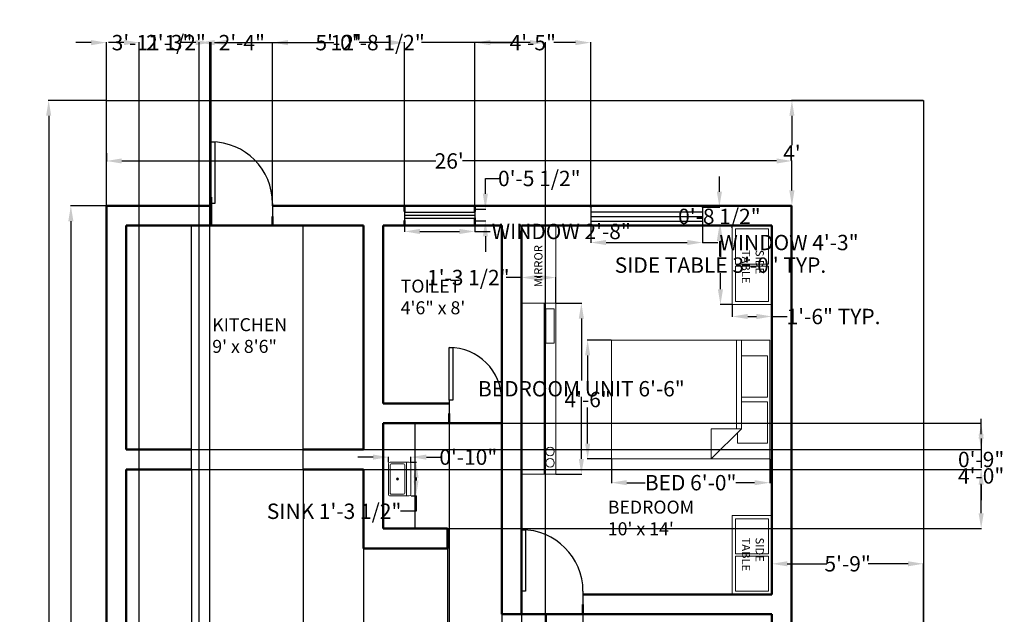
# Model space of a CAD drawing. Units: inches. Extents: x 164 to 612, y 17 to 606.
# Tile 3 of 3: x 164 to 612, y 335 to 606. Entities that reach past the tile are written whole.
import ezdxf

# ---------------------------------------------------------------- set-up
doc = ezdxf.new("R2010")
doc.units = ezdxf.units.IN
doc.header["$MEASUREMENT"] = 0
for name, color, linetype, lineweight in [('A-ANNO-DIMS', 2, 'Continuous', 18), ('A-ANNO-TEXT', 7, 'Continuous', 18), ('A-AREA-IDEN', 7, 'Continuous', 25), ('A-DOOR', 4, 'Continuous', 25), ('A-FLOR-CASE', 9, 'Continuous', 25), ('A-FLOR-FIXT', 9, 'Continuous', 18), ('A-FLOR-STRS', 7, 'Continuous', 25), ('A-FURN', 8, 'Continuous', 18), ('A-GLAZ', 4, 'Continuous', 25), ('A-WALL', 7, 'Continuous', 50), ('C-PROP', 3, 'Continuous', 25)]:
    doc.layers.add(name, color=color, linetype=linetype, lineweight=lineweight)
doc.styles.get("Standard").update_dxf_attribs({"font": 'arial.ttf'})
doc.dimstyles.get("Standard").update_dxf_attribs({"dimtxt": 7, "dimasz": 7, "dimexe": 0.18, "dimexo": 0.0625, "dimgap": 0.09, "dimtad": 0, "dimtih": 1, "dimtoh": 1, "dimdec": 0, "dimzin": 0, "dimdsep": 46, "dimlunit": 3, "dimtxsty": 'Standard', "dimcen": 0.09, "dimadec": 0, "dimazin": 0, "dimtfac": 1, "dimtdec": 0, "dimtofl": 0, "dimtmove": 0, "dimatfit": 3, "dimfxl": 1, "dimtolj": 1, "dimtzin": 0, "dimarcsym": 0})

# ---------------------------------------------------------------- blocks, each defined once
blk = doc.blocks.new('Bed - Queen')
for p, q in [((0, -80.00003), (0, 0)), ((0, 0), (59.99999, 0)), ((59.99999, 0), (59.99999, -80.00003)), ((7.99999, -1.2), (28.79998, -1.2)), ((7.99999, -14.4), (7.99999, -1.2)), ((28.79998, -1.2), (28.79998, -14.4)), ((31.19999, -1.2), (51.99999, -1.2)), ((31.19999, -14.4), (31.19999, -1.2)), ((51.99999, -1.2), (51.99999, -16.4)), ((0, -14.4), (44.8, -14.4)), ((59.99999, -29.6), (44.8, -14.4)), ((44.8, -14.4), (44.8, -29.6)), ((44.8, -16.8), (0, -16.8)), ((51.99999, -16.4), (46.79936, -16.4)), ((44.8, -29.6), (59.99999, -29.6)), ((59.99999, -80.00003), (0, -80.00003))]:
    blk.add_line(p, q)
blk = doc.blocks.new('*U8')
for p, q in [((0, 0), (0, -6)), ((28, 0), (28, -6))]:
    blk.add_line(p, q)
blk.add_lwpolyline([(0, 0), (0, 28), (1.75, 28), (1.75, 0)], close=True)
blk.add_arc((0, 0), 28, 0, 90)
blk = doc.blocks.new('Range Hood - 30 in front')
blk.add_line((0, -4), (30.0001, -4))
for points in [[(0, -6), (0, 0), (30.0001, 0), (30.0001, -6)], [(23, -5.75), (23, -4.25), (29, -4.25), (29, -5.75)]]:
    blk.add_lwpolyline(points, close=True)
for centre in [(2, -5), (4, -5)]:
    blk.add_circle(centre, 0.75)
blk = doc.blocks.new('Wall Cabinet - 18 x 36 in front')
for p, q in [((17.5, -1.5), (17.5, -16.5)), ((18.5, -16.5), (18.5, -1.5))]:
    blk.add_line(p, q)
blk.add_lwpolyline([(0, -18), (0, 0), (36, 0), (36, -18)], close=True)
for points in [[(17.5, -16.5), (1.5, -16.5), (1.5, -1.5), (17.5, -1.5)], [(18.5, -1.5), (34.5, -1.5), (34.5, -16.5), (18.5, -16.5)]]:
    blk.add_lwpolyline(points)
blk = doc.blocks.new('*U13')
for p, q in [((0, 0), (0, -6)), ((24, 0), (24, -6))]:
    blk.add_line(p, q)
blk.add_lwpolyline([(0, 0), (0, 24), (1.75, 24), (1.75, 0)], close=True)
blk.add_arc((0, 0), 24, 0, 90)
blk = doc.blocks.new('Sink-single - 30 in top')
blk.add_line((-15, -3.999996), (15, -3.999996))
for points in [[(-13.5, 0), (13.5, 0)], [(-15, -18.499996), (-15, -1.5)], [(-13.5, -17.499996), (-13.5, -6.499996)], [(-12.5, -5.499996), (12.5, -5.499996)], [(13.5, -6.499996), (13.5, -17.499996)], [(15, -1.5), (15, -18.499996)], [(13.5, -19.999996), (-13.5, -19.999996)], [(12.5, -18.499996), (-12.5, -18.499996)]]:
    blk.add_lwpolyline(points)
for radius in [1, 0.5]:
    blk.add_circle((0, -11.999996), radius)
for centre, radius, start, end in [((-13.5, -1.5), 1.5, 90, 180), ((-12.5, -6.499996), 1, 90, 180), ((12.5, -6.499996), 1, 0, 90), ((13.5, -1.5), 1.5, 0, 90), ((-12.5, -17.499996), 1, 180, 270), ((12.5, -17.499996), 1, 270, 0), ((-13.5, -18.499996), 1.5, 180, 270), ((13.5, -18.499996), 1.5, 270, 0)]:
    blk.add_arc(centre, radius, start, end)
blk = doc.blocks.new('Window - Wood Frame 36 in. Wide plan')
for p, q in [((0, 6), (0, 0)), ((0, 4.5), (36, 4.5)), ((36, 6), (36, 0)), ((0, 3), (36, 3)), ((0, 1.5), (36, 1.5))]:
    blk.add_line(p, q)
blk = doc.blocks.new('*D14')
at = {"layer": 'A-ANNO-DIMS', "color": 0, "lineweight": -2, "transparency": 16777216}
for p, q in [((575.51, 569.38), (515.53, 569.38)), ((515.71, 562.38), (515.71, 548.97)), ((515.71, 528.38), (515.71, 541.79)), ((515.63, 521.38), (515.89, 521.38))]:
    blk.add_line(p, q, dxfattribs=at)
at = {"layer": 'A-ANNO-DIMS', "color": 0, "transparency": 16777216}
for points in [[(514.54, 562.38), (516.87, 562.38), (515.71, 569.38)], [(514.54, 528.38), (516.87, 528.38), (515.71, 521.38)]]:
    blk.add_solid(points, dxfattribs=at)
at = {"layer": 'Defpoints', "color": 0, "transparency": 16777216}
for p in [(515.71, 569.38), (575.57, 569.38), (515.57, 521.38)]:
    blk.add_point(p, dxfattribs=at)
at = {"layer": 'A-ANNO-DIMS', "color": 0, "transparency": 16777216, "insert": (515.71, 545.38), "char_height": 7, "attachment_point": 5}
blk.add_mtext("\\A1;4'", dxfattribs=at)
blk = doc.blocks.new('*D15')
at = {"layer": 'A-ANNO-DIMS', "color": 0, "lineweight": -2, "transparency": 16777216}
for p, q in [((203.57, 545.32), (203.57, 541.61)), ((210.57, 541.79), (353.55, 541.79)), ((508.71, 541.79), (365.73, 541.79)), ((515.71, 541.85), (515.71, 541.97))]:
    blk.add_line(p, q, dxfattribs=at)
at = {"layer": 'A-ANNO-DIMS', "color": 0, "transparency": 16777216}
for points in [[(210.57, 542.96), (210.57, 540.62), (203.57, 541.79)], [(508.71, 542.96), (508.71, 540.62), (515.71, 541.79)]]:
    blk.add_solid(points, dxfattribs=at)
at = {"layer": 'Defpoints', "color": 0, "transparency": 16777216}
for p in [(203.57, 545.38), (515.71, 541.79), (515.71, 541.79)]:
    blk.add_point(p, dxfattribs=at)
at = {"layer": 'A-ANNO-DIMS', "color": 0, "transparency": 16777216, "insert": (359.64, 541.79), "char_height": 7, "attachment_point": 5}
blk.add_mtext("\\A1;26'", dxfattribs=at)
blk = doc.blocks.new('*D19')
at = {"layer": 'A-ANNO-DIMS', "color": 0, "lineweight": -2, "transparency": 16777216}
for p, q in [((506.57, 344.44), (506.57, 358.56)), ((513.57, 358.38), (531.68, 358.38)), ((568.57, 358.38), (550.46, 358.38)), ((575.57, 311.44), (575.57, 358.56))]:
    blk.add_line(p, q, dxfattribs=at)
at = {"layer": 'A-ANNO-DIMS', "color": 0, "transparency": 16777216}
for points in [[(513.57, 359.55), (513.57, 357.22), (506.57, 358.38)], [(568.57, 359.55), (568.57, 357.22), (575.57, 358.38)]]:
    blk.add_solid(points, dxfattribs=at)
at = {"layer": 'Defpoints', "color": 0, "transparency": 16777216}
for p in [(575.57, 358.38), (506.57, 344.38), (575.57, 311.38)]:
    blk.add_point(p, dxfattribs=at)
at = {"layer": 'A-ANNO-DIMS', "color": 0, "transparency": 16777216, "insert": (541.07, 358.38), "char_height": 7, "attachment_point": 5}
blk.add_mtext('\\A1;5\'-9"', dxfattribs=at)
blk = doc.blocks.new('*D20')
at = {"layer": 'A-ANNO-DIMS', "color": 0, "lineweight": -2, "transparency": 16777216}
for p, q in [((212.57, 401.32), (212.57, 325.08)), ((383.57, 335.32), (383.57, 325.08)), ((219.57, 325.26), (286.29, 325.26)), ((376.57, 325.26), (309.85, 325.26))]:
    blk.add_line(p, q, dxfattribs=at)
at = {"layer": 'A-ANNO-DIMS', "color": 0, "transparency": 16777216}
for points in [[(219.57, 326.42), (219.57, 324.09), (212.57, 325.26)], [(376.57, 326.42), (376.57, 324.09), (383.57, 325.26)]]:
    blk.add_solid(points, dxfattribs=at)
at = {"layer": 'Defpoints', "color": 0, "transparency": 16777216}
for p in [(212.57, 401.38), (383.57, 335.38), (212.57, 325.26)]:
    blk.add_point(p, dxfattribs=at)
at = {"layer": 'A-ANNO-DIMS', "color": 0, "transparency": 16777216, "insert": (298.07, 325.26), "char_height": 7, "attachment_point": 5}
blk.add_mtext('\\A1;14\'-3"', dxfattribs=at)
blk = doc.blocks.new('*D21')
at = {"layer": 'A-ANNO-DIMS', "color": 0, "lineweight": -2, "transparency": 16777216}
for p, q in [((227.33, 521.38), (187.19, 521.38)), ((187.37, 514.38), (187.37, 321.05)), ((187.37, 120.38), (187.37, 313.71)), ((217.32, 113.38), (187.19, 113.38))]:
    blk.add_line(p, q, dxfattribs=at)
at = {"layer": 'A-ANNO-DIMS', "color": 0, "transparency": 16777216}
for points in [[(186.2, 514.38), (188.54, 514.38), (187.37, 521.38)], [(186.2, 120.38), (188.54, 120.38), (187.37, 113.38)]]:
    blk.add_solid(points, dxfattribs=at)
at = {"layer": 'Defpoints', "color": 0, "transparency": 16777216}
for p in [(227.39, 521.38), (187.37, 113.38), (217.38, 113.38)]:
    blk.add_point(p, dxfattribs=at)
at = {"layer": 'A-ANNO-DIMS', "color": 0, "transparency": 16777216, "insert": (187.37, 317.38), "char_height": 7, "attachment_point": 5}
blk.add_mtext("\\A1;34'", dxfattribs=at)
blk = doc.blocks.new('*D22')
at = {"layer": 'A-ANNO-DIMS', "color": 0, "lineweight": -2, "transparency": 16777216}
for p, q in [((488.51, 512.38), (482.99, 512.38)), ((483.17, 505.38), (483.17, 498.09)), ((483.17, 483.38), (483.17, 490.67)), ((488.51, 476.38), (482.99, 476.38))]:
    blk.add_line(p, q, dxfattribs=at)
at = {"layer": 'A-ANNO-DIMS', "color": 0, "transparency": 16777216}
for points in [[(482, 505.38), (484.34, 505.38), (483.17, 512.38)], [(482, 483.38), (484.34, 483.38), (483.17, 476.38)]]:
    blk.add_solid(points, dxfattribs=at)
at = {"layer": 'Defpoints', "color": 0, "transparency": 16777216}
for p in [(488.57, 512.38), (483.17, 476.38), (488.57, 476.38)]:
    blk.add_point(p, dxfattribs=at)
at = {"layer": 'A-ANNO-DIMS', "color": 0, "transparency": 16777216, "insert": (483.17, 494.38), "char_height": 7, "attachment_point": 5}
blk.add_mtext('\\A1;SIDE TABLE 3\'-0" TYP.', dxfattribs=at)
blk = doc.blocks.new('*D23')
at = {"layer": 'A-ANNO-DIMS', "color": 0, "lineweight": -2, "transparency": 16777216}
for p, q in [((488.57, 476.32), (488.57, 470.8)), ((506.57, 476.32), (506.57, 470.8)), ((495.57, 470.98), (499.57, 470.98)), ((506.57, 470.98), (513.57, 470.98))]:
    blk.add_line(p, q, dxfattribs=at)
at = {"layer": 'A-ANNO-DIMS', "color": 0, "transparency": 16777216}
for points in [[(495.57, 472.15), (495.57, 469.81), (488.57, 470.98)], [(499.57, 472.15), (499.57, 469.81), (506.57, 470.98)]]:
    blk.add_solid(points, dxfattribs=at)
at = {"layer": 'Defpoints', "color": 0, "transparency": 16777216}
for p in [(488.57, 476.38), (506.57, 476.38), (506.57, 470.98)]:
    blk.add_point(p, dxfattribs=at)
at = {"layer": 'A-ANNO-DIMS', "color": 0, "transparency": 16777216, "insert": (534.66, 470.98), "char_height": 7, "attachment_point": 5}
blk.add_mtext('\\A1;1\'-6" TYP.', dxfattribs=at)
blk = doc.blocks.new('*D24')
at = {"layer": 'A-ANNO-DIMS', "color": 0, "lineweight": -2, "transparency": 16777216}
for p, q in [((339.33, 514.43), (339.33, 509.52)), ((371.32, 514.43), (371.32, 509.52)), ((346.33, 509.7), (364.32, 509.7)), ((371.32, 509.7), (378.32, 509.7))]:
    blk.add_line(p, q, dxfattribs=at)
at = {"layer": 'A-ANNO-DIMS', "color": 0, "transparency": 16777216}
for points in [[(346.33, 510.86), (346.33, 508.53), (339.33, 509.7)], [(364.32, 510.86), (364.32, 508.53), (371.32, 509.7)]]:
    blk.add_solid(points, dxfattribs=at)
at = {"layer": 'Defpoints', "color": 0, "transparency": 16777216}
for p in [(339.33, 514.49), (371.32, 514.49), (371.32, 509.7)]:
    blk.add_point(p, dxfattribs=at)
at = {"layer": 'A-ANNO-DIMS', "color": 0, "transparency": 16777216, "insert": (410.67, 509.7), "char_height": 7, "attachment_point": 5}
blk.add_mtext('\\A1;WINDOW 2\'-8"', dxfattribs=at)
blk = doc.blocks.new('*D25')
at = {"layer": 'A-ANNO-DIMS', "color": 0, "lineweight": -2, "transparency": 16777216}
for p, q in [((376.12, 526.83), (376.12, 533.83)), ((376.12, 533.83), (383.12, 533.83)), ((371.38, 519.83), (376.3, 519.83)), ((371.38, 514.49), (376.3, 514.49)), ((376.12, 507.49), (376.12, 500.49))]:
    blk.add_line(p, q, dxfattribs=at)
at = {"layer": 'A-ANNO-DIMS', "color": 0, "transparency": 16777216}
for points in [[(374.95, 526.83), (377.28, 526.83), (376.12, 519.83)], [(374.95, 507.49), (377.28, 507.49), (376.12, 514.49)]]:
    blk.add_solid(points, dxfattribs=at)
at = {"layer": 'Defpoints', "color": 0, "transparency": 16777216}
for p in [(371.32, 519.83), (376.12, 519.83), (371.32, 514.49)]:
    blk.add_point(p, dxfattribs=at)
at = {"layer": 'A-ANNO-DIMS', "color": 0, "transparency": 16777216, "insert": (400.67, 533.83), "char_height": 7, "attachment_point": 5}
blk.add_mtext('\\A1;0\'-5 1/2"', dxfattribs=at)
blk = doc.blocks.new('*D26')
at = {"layer": 'A-ANNO-DIMS', "color": 0, "lineweight": -2, "transparency": 16777216}
for p, q in [((424.1, 512.24), (424.1, 504.48)), ((475.04, 512.24), (475.04, 504.48)), ((431.1, 504.66), (468.04, 504.66)), ((475.04, 504.66), (482.04, 504.66))]:
    blk.add_line(p, q, dxfattribs=at)
at = {"layer": 'A-ANNO-DIMS', "color": 0, "transparency": 16777216}
for points in [[(431.1, 505.83), (431.1, 503.49), (424.1, 504.66)], [(468.04, 505.83), (468.04, 503.49), (475.04, 504.66)]]:
    blk.add_solid(points, dxfattribs=at)
at = {"layer": 'Defpoints', "color": 0, "transparency": 16777216}
for p in [(424.1, 512.3), (475.04, 512.3), (475.04, 504.66)]:
    blk.add_point(p, dxfattribs=at)
at = {"layer": 'A-ANNO-DIMS', "color": 0, "transparency": 16777216, "insert": (514.39, 504.66), "char_height": 7, "attachment_point": 5}
blk.add_mtext('\\A1;WINDOW 4\'-3"', dxfattribs=at)
blk = doc.blocks.new('*D27')
at = {"layer": 'A-ANNO-DIMS', "color": 0, "lineweight": -2, "transparency": 16777216}
for p, q in [((482.68, 527.79), (482.68, 534.79)), ((475.1, 520.79), (482.86, 520.79)), ((475.1, 512.3), (482.86, 512.3)), ((482.68, 505.3), (482.68, 498.3))]:
    blk.add_line(p, q, dxfattribs=at)
at = {"layer": 'A-ANNO-DIMS', "color": 0, "transparency": 16777216}
for points in [[(481.51, 527.79), (483.84, 527.79), (482.68, 520.79)], [(481.51, 505.3), (483.84, 505.3), (482.68, 512.3)]]:
    blk.add_solid(points, dxfattribs=at)
at = {"layer": 'Defpoints', "color": 0, "transparency": 16777216}
for p in [(475.04, 520.79), (482.68, 520.79), (475.04, 512.3)]:
    blk.add_point(p, dxfattribs=at)
at = {"layer": 'A-ANNO-DIMS', "color": 0, "transparency": 16777216, "insert": (482.68, 516.55), "char_height": 7, "attachment_point": 5}
blk.add_mtext('\\A1;0\'-8 1/2"', dxfattribs=at)
blk = doc.blocks.new('*D28')
at = {"layer": 'A-ANNO-DIMS', "color": 0, "lineweight": -2, "transparency": 16777216}
for p, q in [((433.51, 406.07), (433.51, 395.13)), ((505.67, 406.07), (505.67, 395.13)), ((440.51, 395.31), (448.94, 395.31)), ((498.67, 395.31), (490.24, 395.31))]:
    blk.add_line(p, q, dxfattribs=at)
at = {"layer": 'A-ANNO-DIMS', "color": 0, "transparency": 16777216}
for points in [[(440.51, 396.48), (440.51, 394.14), (433.51, 395.31)], [(498.67, 396.48), (498.67, 394.14), (505.67, 395.31)]]:
    blk.add_solid(points, dxfattribs=at)
at = {"layer": 'Defpoints', "color": 0, "transparency": 16777216}
for p in [(433.51, 406.14), (505.67, 406.14), (505.67, 395.31)]:
    blk.add_point(p, dxfattribs=at)
at = {"layer": 'A-ANNO-DIMS', "color": 0, "transparency": 16777216, "insert": (469.59, 395.31), "char_height": 7, "attachment_point": 5}
blk.add_mtext('\\A1;BED 6\'-0"', dxfattribs=at)
blk = doc.blocks.new('*D29')
at = {"layer": 'A-ANNO-DIMS', "color": 0, "lineweight": -2, "transparency": 16777216}
for p, q in [((433.45, 460.25), (422.51, 460.25)), ((422.69, 453.25), (422.69, 436.86)), ((422.69, 413.14), (422.69, 429.53)), ((433.45, 406.14), (422.51, 406.14))]:
    blk.add_line(p, q, dxfattribs=at)
at = {"layer": 'A-ANNO-DIMS', "color": 0, "transparency": 16777216}
for points in [[(421.52, 453.25), (423.85, 453.25), (422.69, 460.25)], [(421.52, 413.14), (423.85, 413.14), (422.69, 406.14)]]:
    blk.add_solid(points, dxfattribs=at)
at = {"layer": 'Defpoints', "color": 0, "transparency": 16777216}
for p in [(433.51, 460.25), (422.69, 406.14), (433.51, 406.14)]:
    blk.add_point(p, dxfattribs=at)
at = {"layer": 'A-ANNO-DIMS', "color": 0, "transparency": 16777216, "insert": (422.69, 433.19), "char_height": 7, "attachment_point": 5}
blk.add_mtext('\\A1;4\'-6"', dxfattribs=at)
blk = doc.blocks.new('*D38')
at = {"layer": 'A-ANNO-DIMS', "color": 0, "lineweight": -2, "transparency": 16777216}
for p, q in [((408.21, 477.03), (420.01, 477.03)), ((419.83, 470.03), (419.83, 441.79)), ((419.83, 406.13), (419.83, 434.37)), ((408.21, 399.13), (420.01, 399.13))]:
    blk.add_line(p, q, dxfattribs=at)
at = {"layer": 'A-ANNO-DIMS', "color": 0, "transparency": 16777216}
for points in [[(418.67, 470.03), (421, 470.03), (419.83, 477.03)], [(418.67, 406.13), (421, 406.13), (419.83, 399.13)]]:
    blk.add_solid(points, dxfattribs=at)
at = {"layer": 'Defpoints', "color": 0, "transparency": 16777216}
for p in [(408.15, 477.03), (419.83, 477.03), (408.15, 399.13)]:
    blk.add_point(p, dxfattribs=at)
at = {"layer": 'A-ANNO-DIMS', "color": 0, "transparency": 16777216, "insert": (419.83, 438.08), "char_height": 7, "attachment_point": 5}
blk.add_mtext('\\A1;BEDROOM UNIT 6\'-6"', dxfattribs=at)
blk = doc.blocks.new('*D39')
at = {"layer": 'A-ANNO-DIMS', "color": 0, "lineweight": -2, "transparency": 16777216}
for p, q in [((392.57, 488.71), (385.57, 488.71)), ((392.57, 477.09), (392.57, 488.89)), ((401.15, 488.71), (399.57, 488.71)), ((408.15, 477.09), (408.15, 488.89))]:
    blk.add_line(p, q, dxfattribs=at)
at = {"layer": 'A-ANNO-DIMS', "color": 0, "transparency": 16777216}
for points in [[(399.57, 489.88), (399.57, 487.55), (392.57, 488.71)], [(401.15, 489.88), (401.15, 487.55), (408.15, 488.71)]]:
    blk.add_solid(points, dxfattribs=at)
at = {"layer": 'Defpoints', "color": 0, "transparency": 16777216}
for p in [(392.57, 488.71), (392.57, 477.03), (408.15, 477.03)]:
    blk.add_point(p, dxfattribs=at)
at = {"layer": 'A-ANNO-DIMS', "color": 0, "transparency": 16777216, "insert": (368.35, 488.71), "char_height": 7, "attachment_point": 5}
blk.add_mtext('\\A1;1\'-3 1/2"', dxfattribs=at)
blk = doc.blocks.new('*D40')
at = {"layer": 'A-ANNO-DIMS', "color": 0, "lineweight": -2, "transparency": 16777216}
for p, q in [((342.3, 404.65), (344.72, 404.65)), ((344.54, 397.65), (344.54, 396.29)), ((342.3, 389.29), (344.72, 389.29)), ((344.54, 389.29), (344.54, 382.29)), ((344.54, 382.29), (337.54, 382.29))]:
    blk.add_line(p, q, dxfattribs=at)
at = {"layer": 'A-ANNO-DIMS', "color": 0, "transparency": 16777216}
for points in [[(343.38, 397.65), (345.71, 397.65), (344.54, 404.65)], [(343.38, 396.29), (345.71, 396.29), (344.54, 389.29)]]:
    blk.add_solid(points, dxfattribs=at)
at = {"layer": 'Defpoints', "color": 0, "transparency": 16777216}
for p in [(342.24, 404.65), (342.24, 389.29), (344.54, 389.29)]:
    blk.add_point(p, dxfattribs=at)
at = {"layer": 'A-ANNO-DIMS', "color": 0, "transparency": 16777216, "insert": (307.24, 382.29), "char_height": 7, "attachment_point": 5}
blk.add_mtext('\\A1;SINK 1\'-3 1/2"', dxfattribs=at)
blk = doc.blocks.new('*D41')
at = {"layer": 'A-ANNO-DIMS', "color": 0, "lineweight": -2, "transparency": 16777216}
for p, q in [((325, 406.95), (318, 406.95)), ((332, 404.71), (332, 407.13)), ((342.24, 404.71), (342.24, 407.13)), ((349.24, 406.95), (356.24, 406.95))]:
    blk.add_line(p, q, dxfattribs=at)
at = {"layer": 'A-ANNO-DIMS', "color": 0, "transparency": 16777216}
for points in [[(325, 408.12), (325, 405.79), (332, 406.95)], [(349.24, 408.12), (349.24, 405.79), (342.24, 406.95)]]:
    blk.add_solid(points, dxfattribs=at)
at = {"layer": 'Defpoints', "color": 0, "transparency": 16777216}
for p in [(332, 404.65), (342.24, 406.95), (342.24, 404.65)]:
    blk.add_point(p, dxfattribs=at)
at = {"layer": 'A-ANNO-DIMS', "color": 0, "transparency": 16777216, "insert": (368.35, 406.95), "char_height": 7, "attachment_point": 5}
blk.add_mtext('\\A1;0\'-10"', dxfattribs=at)
blk = doc.blocks.new('*D43')
at = {"layer": 'A-ANNO-DIMS', "color": 0, "lineweight": -2, "transparency": 16777216}
for p, q in [((203.51, 569.38), (177.09, 569.38)), ((177.27, 562.38), (177.27, 315.05)), ((177.27, 60.38), (177.27, 307.71)), ((203.51, 53.38), (177.09, 53.38))]:
    blk.add_line(p, q, dxfattribs=at)
at = {"layer": 'A-ANNO-DIMS', "color": 0, "transparency": 16777216}
for points in [[(176.1, 562.38), (178.44, 562.38), (177.27, 569.38)], [(176.1, 60.38), (178.44, 60.38), (177.27, 53.38)]]:
    blk.add_solid(points, dxfattribs=at)
at = {"layer": 'Defpoints', "color": 0, "transparency": 16777216}
for p in [(177.27, 569.38), (203.57, 569.38), (203.57, 53.38)]:
    blk.add_point(p, dxfattribs=at)
at = {"layer": 'A-ANNO-DIMS', "color": 0, "transparency": 16777216, "insert": (177.27, 311.38), "char_height": 7, "attachment_point": 5}
blk.add_mtext('\\A1;43\'-0"', dxfattribs=at)
blk = doc.blocks.new('*D44')
at = {"layer": 'A-ANNO-DIMS', "color": 0, "lineweight": -2, "transparency": 16777216}
for p, q in [((196.57, 595.68), (189.57, 595.68)), ((203.57, 521.44), (203.57, 595.86)), ((251.22, 521.44), (251.22, 595.86)), ((258.22, 595.68), (265.22, 595.68))]:
    blk.add_line(p, q, dxfattribs=at)
at = {"layer": 'A-ANNO-DIMS', "color": 0, "transparency": 16777216}
for points in [[(196.57, 596.85), (196.57, 594.51), (203.57, 595.68)], [(258.22, 596.85), (258.22, 594.51), (251.22, 595.68)]]:
    blk.add_solid(points, dxfattribs=at)
at = {"layer": 'Defpoints', "color": 0, "transparency": 16777216}
for p in [(251.22, 595.68), (203.57, 521.38), (251.22, 521.38)]:
    blk.add_point(p, dxfattribs=at)
at = {"layer": 'A-ANNO-DIMS', "color": 0, "transparency": 16777216, "insert": (227.39, 595.68), "char_height": 7, "attachment_point": 5}
blk.add_mtext('\\A1;3\'-11 1/2"', dxfattribs=at)
blk = doc.blocks.new('*D45')
at = {"layer": 'A-ANNO-DIMS', "color": 0, "lineweight": -2, "transparency": 16777216}
for p, q in [((244.22, 595.68), (237.22, 595.68)), ((251.22, 521.44), (251.22, 595.86)), ((279.22, 521.44), (279.22, 595.86)), ((286.22, 595.68), (293.22, 595.68))]:
    blk.add_line(p, q, dxfattribs=at)
at = {"layer": 'A-ANNO-DIMS', "color": 0, "transparency": 16777216}
for points in [[(244.22, 596.85), (244.22, 594.51), (251.22, 595.68)], [(286.22, 596.85), (286.22, 594.51), (279.22, 595.68)]]:
    blk.add_solid(points, dxfattribs=at)
at = {"layer": 'Defpoints', "color": 0, "transparency": 16777216}
for p in [(279.22, 595.68), (251.22, 521.38), (279.22, 521.38)]:
    blk.add_point(p, dxfattribs=at)
at = {"layer": 'A-ANNO-DIMS', "color": 0, "transparency": 16777216, "insert": (265.22, 595.68), "char_height": 7, "attachment_point": 5}
blk.add_mtext('\\A1;2\'-4"', dxfattribs=at)
blk = doc.blocks.new('*D46')
at = {"layer": 'A-ANNO-DIMS', "color": 0, "lineweight": -2, "transparency": 16777216}
for p, q in [((279.22, 521.44), (279.22, 595.86)), ((286.22, 595.68), (299.88, 595.68)), ((332.33, 595.68), (318.67, 595.68)), ((339.33, 521.44), (339.33, 595.86))]:
    blk.add_line(p, q, dxfattribs=at)
at = {"layer": 'A-ANNO-DIMS', "color": 0, "transparency": 16777216}
for points in [[(286.22, 596.85), (286.22, 594.51), (279.22, 595.68)], [(332.33, 596.85), (332.33, 594.51), (339.33, 595.68)]]:
    blk.add_solid(points, dxfattribs=at)
at = {"layer": 'Defpoints', "color": 0, "transparency": 16777216}
for p in [(339.33, 595.68), (279.22, 521.38), (339.33, 521.38)]:
    blk.add_point(p, dxfattribs=at)
at = {"layer": 'A-ANNO-DIMS', "color": 0, "transparency": 16777216, "insert": (309.27, 595.68), "char_height": 7, "attachment_point": 5}
blk.add_mtext('\\A1;5\'-0"', dxfattribs=at)
blk = doc.blocks.new('*D47')
at = {"layer": 'A-ANNO-DIMS', "color": 0, "lineweight": -2, "transparency": 16777216}
for p, q in [((371.32, 521.44), (371.32, 595.86)), ((378.32, 595.68), (388.18, 595.68)), ((417.1, 595.68), (407.25, 595.68)), ((424.1, 521.44), (424.1, 595.86))]:
    blk.add_line(p, q, dxfattribs=at)
at = {"layer": 'A-ANNO-DIMS', "color": 0, "transparency": 16777216}
for points in [[(378.32, 596.85), (378.32, 594.51), (371.32, 595.68)], [(417.1, 596.85), (417.1, 594.51), (424.1, 595.68)]]:
    blk.add_solid(points, dxfattribs=at)
at = {"layer": 'Defpoints', "color": 0, "transparency": 16777216}
for p in [(424.1, 595.68), (371.32, 521.38), (424.1, 521.38)]:
    blk.add_point(p, dxfattribs=at)
at = {"layer": 'A-ANNO-DIMS', "color": 0, "transparency": 16777216, "insert": (397.71, 595.68), "char_height": 7, "attachment_point": 5}
blk.add_mtext('\\A1;4\'-5"', dxfattribs=at)
blk = doc.blocks.new('*D49')
at = {"layer": 'A-ANNO-DIMS', "color": 0, "lineweight": -2, "transparency": 16777216}
for p, q in [((392.57, 344.32), (392.57, 26.9)), ((420.57, 344.32), (420.57, 26.9)), ((385.57, 27.08), (378.57, 27.08)), ((427.57, 27.08), (434.57, 27.08))]:
    blk.add_line(p, q, dxfattribs=at)
at = {"layer": 'A-ANNO-DIMS', "color": 0, "transparency": 16777216}
for points in [[(385.57, 28.25), (385.57, 25.91), (392.57, 27.08)], [(427.57, 28.25), (427.57, 25.91), (420.57, 27.08)]]:
    blk.add_solid(points, dxfattribs=at)
at = {"layer": 'Defpoints', "color": 0, "transparency": 16777216}
for p in [(392.57, 344.38), (420.57, 344.38), (420.57, 27.08)]:
    blk.add_point(p, dxfattribs=at)
at = {"layer": 'A-ANNO-DIMS', "color": 0, "transparency": 16777216, "insert": (406.57, 27.08), "char_height": 7, "attachment_point": 5}
blk.add_mtext('\\A1;2\'-4"', dxfattribs=at)
blk = doc.blocks.new('*D50')
at = {"layer": 'A-ANNO-DIMS', "color": 0, "lineweight": -2, "transparency": 16777216}
for p, q in [((359.57, 422.32), (359.57, 26.9)), ((383.57, 422.32), (383.57, 26.9)), ((352.57, 27.08), (345.57, 27.08)), ((390.57, 27.08), (397.57, 27.08))]:
    blk.add_line(p, q, dxfattribs=at)
at = {"layer": 'A-ANNO-DIMS', "color": 0, "transparency": 16777216}
for points in [[(352.57, 28.25), (352.57, 25.91), (359.57, 27.08)], [(390.57, 28.25), (390.57, 25.91), (383.57, 27.08)]]:
    blk.add_solid(points, dxfattribs=at)
at = {"layer": 'Defpoints', "color": 0, "transparency": 16777216}
for p in [(359.57, 422.38), (383.57, 422.38), (383.57, 27.08)]:
    blk.add_point(p, dxfattribs=at)
at = {"layer": 'A-ANNO-DIMS', "color": 0, "transparency": 16777216, "insert": (371.57, 27.08), "char_height": 7, "attachment_point": 5}
blk.add_mtext('\\A1;2\'-0"', dxfattribs=at)
blk = doc.blocks.new('*D54')
at = {"layer": 'A-ANNO-DIMS', "color": 0, "lineweight": -2, "transparency": 16777216}
for p, q in [((212.57, 401.32), (212.57, 26.9)), ((242.38, 401.32), (242.38, 26.9)), ((205.57, 27.08), (198.57, 27.08)), ((249.38, 27.08), (256.38, 27.08))]:
    blk.add_line(p, q, dxfattribs=at)
at = {"layer": 'A-ANNO-DIMS', "color": 0, "transparency": 16777216}
for points in [[(205.57, 28.25), (205.57, 25.91), (212.57, 27.08)], [(249.38, 28.25), (249.38, 25.91), (242.38, 27.08)]]:
    blk.add_solid(points, dxfattribs=at)
at = {"layer": 'Defpoints', "color": 0, "transparency": 16777216}
for p in [(212.57, 401.38), (242.38, 401.38), (242.38, 27.08)]:
    blk.add_point(p, dxfattribs=at)
at = {"layer": 'A-ANNO-DIMS', "color": 0, "transparency": 16777216, "insert": (227.47, 27.08), "char_height": 7, "attachment_point": 5}
blk.add_mtext('\\A1;2\'-6"', dxfattribs=at)
blk = doc.blocks.new('*D55')
at = {"layer": 'A-ANNO-DIMS', "color": 0, "lineweight": -2, "transparency": 16777216}
for p, q in [((242.38, 401.32), (242.38, 26.9)), ((293.15, 401.32), (293.15, 26.9)), ((249.38, 27.08), (258.23, 27.08)), ((286.15, 27.08), (277.3, 27.08))]:
    blk.add_line(p, q, dxfattribs=at)
at = {"layer": 'A-ANNO-DIMS', "color": 0, "transparency": 16777216}
for points in [[(249.38, 28.25), (249.38, 25.91), (242.38, 27.08)], [(286.15, 28.25), (286.15, 25.91), (293.15, 27.08)]]:
    blk.add_solid(points, dxfattribs=at)
at = {"layer": 'Defpoints', "color": 0, "transparency": 16777216}
for p in [(242.38, 401.38), (293.15, 401.38), (293.15, 27.08)]:
    blk.add_point(p, dxfattribs=at)
at = {"layer": 'A-ANNO-DIMS', "color": 0, "transparency": 16777216, "insert": (267.76, 27.08), "char_height": 7, "attachment_point": 5}
blk.add_mtext('\\A1;4\'-3"', dxfattribs=at)
blk = doc.blocks.new('*D56')
at = {"layer": 'A-ANNO-DIMS', "color": 0, "lineweight": -2, "transparency": 16777216}
for p, q in [((250.72, 154.11), (250.72, 595.86)), ((257.72, 595.68), (307.15, 595.68)), ((396.46, 595.68), (347.03, 595.68)), ((403.46, 154.11), (403.46, 595.86))]:
    blk.add_line(p, q, dxfattribs=at)
at = {"layer": 'A-ANNO-DIMS', "color": 0, "transparency": 16777216}
for points in [[(257.72, 596.85), (257.72, 594.51), (250.72, 595.68)], [(396.46, 596.85), (396.46, 594.51), (403.46, 595.68)]]:
    blk.add_solid(points, dxfattribs=at)
at = {"layer": 'Defpoints', "color": 0, "transparency": 16777216}
for p in [(403.46, 595.68), (250.72, 154.05), (403.46, 154.05)]:
    blk.add_point(p, dxfattribs=at)
at = {"layer": 'A-ANNO-DIMS', "color": 0, "transparency": 16777216, "insert": (327.09, 595.68), "char_height": 7, "attachment_point": 5}
blk.add_mtext('\\A1;12\'-8 1/2"', dxfattribs=at)
blk = doc.blocks.new('*D57')
at = {"layer": 'A-ANNO-DIMS', "color": 0, "lineweight": -2, "transparency": 16777216}
for p, q in [((211.55, 595.68), (204.55, 595.68)), ((218.55, 245.57), (218.55, 595.86)), ((245.79, 245.57), (245.79, 595.86)), ((252.79, 595.68), (259.79, 595.68))]:
    blk.add_line(p, q, dxfattribs=at)
at = {"layer": 'A-ANNO-DIMS', "color": 0, "transparency": 16777216}
for points in [[(211.55, 596.85), (211.55, 594.51), (218.55, 595.68)], [(252.79, 596.85), (252.79, 594.51), (245.79, 595.68)]]:
    blk.add_solid(points, dxfattribs=at)
at = {"layer": 'Defpoints', "color": 0, "transparency": 16777216}
for p in [(245.79, 595.68), (218.55, 245.51), (245.79, 245.51)]:
    blk.add_point(p, dxfattribs=at)
at = {"layer": 'A-ANNO-DIMS', "color": 0, "transparency": 16777216, "insert": (232.17, 595.68), "char_height": 7, "attachment_point": 5}
blk.add_mtext('\\A1;2\'-3"', dxfattribs=at)
blk = doc.blocks.new('*D58')
at = {"layer": 'A-ANNO-DIMS', "color": 0, "lineweight": -2, "transparency": 16777216}
for p, q in [((601.87, 417.38), (601.87, 424.38)), ((242.44, 410.38), (602.05, 410.38)), ((242.44, 401.38), (602.05, 401.38)), ((601.87, 394.38), (601.87, 387.38))]:
    blk.add_line(p, q, dxfattribs=at)
at = {"layer": 'A-ANNO-DIMS', "color": 0, "transparency": 16777216}
for points in [[(600.7, 417.38), (603.04, 417.38), (601.87, 410.38)], [(600.7, 394.38), (603.04, 394.38), (601.87, 401.38)]]:
    blk.add_solid(points, dxfattribs=at)
at = {"layer": 'Defpoints', "color": 0, "transparency": 16777216}
for p in [(242.38, 410.38), (601.87, 410.38), (242.38, 401.38)]:
    blk.add_point(p, dxfattribs=at)
at = {"layer": 'A-ANNO-DIMS', "color": 0, "transparency": 16777216, "insert": (601.87, 405.88), "char_height": 7, "attachment_point": 5}
blk.add_mtext('\\A1;0\'-9"', dxfattribs=at)
blk = doc.blocks.new('*D59')
at = {"layer": 'A-ANNO-DIMS', "color": 0, "lineweight": -2, "transparency": 16777216}
for p, q in [((344.28, 422.38), (602.05, 422.38)), ((601.87, 415.38), (601.87, 402.04)), ((601.87, 381.38), (601.87, 394.72)), ((344.28, 374.38), (602.05, 374.38))]:
    blk.add_line(p, q, dxfattribs=at)
at = {"layer": 'A-ANNO-DIMS', "color": 0, "transparency": 16777216}
for points in [[(600.7, 415.38), (603.04, 415.38), (601.87, 422.38)], [(600.7, 381.38), (603.04, 381.38), (601.87, 374.38)]]:
    blk.add_solid(points, dxfattribs=at)
at = {"layer": 'Defpoints', "color": 0, "transparency": 16777216}
for p in [(344.22, 422.38), (601.87, 422.38), (344.22, 374.38)]:
    blk.add_point(p, dxfattribs=at)
at = {"layer": 'A-ANNO-DIMS', "color": 0, "transparency": 16777216, "insert": (601.87, 398.38), "char_height": 7, "attachment_point": 5}
blk.add_mtext('\\A1;4\'-0"', dxfattribs=at)
blk = doc.blocks.new('*D60')
at = {"layer": 'A-ANNO-DIMS', "color": 0, "lineweight": -2, "transparency": 16777216}
for p, q in [((320.57, 365.32), (320.57, 26.9)), ((358.87, 365.32), (358.87, 26.9)), ((313.57, 27.08), (306.57, 27.08)), ((365.87, 27.08), (372.87, 27.08))]:
    blk.add_line(p, q, dxfattribs=at)
at = {"layer": 'A-ANNO-DIMS', "color": 0, "transparency": 16777216}
for points in [[(313.57, 28.25), (313.57, 25.91), (320.57, 27.08)], [(365.87, 28.25), (365.87, 25.91), (358.87, 27.08)]]:
    blk.add_solid(points, dxfattribs=at)
at = {"layer": 'Defpoints', "color": 0, "transparency": 16777216}
for p in [(320.57, 365.38), (358.87, 365.38), (358.87, 27.08)]:
    blk.add_point(p, dxfattribs=at)
at = {"layer": 'A-ANNO-DIMS', "color": 0, "transparency": 16777216, "insert": (339.72, 27.08), "char_height": 7, "attachment_point": 5}
blk.add_mtext('\\A1;3\'-2 1/2"', dxfattribs=at)

msp = doc.modelspace()

# ---------------------------------------------------------------- linework, layer by layer
at = {"layer": 'A-FLOR-CASE'}
for p, q in [((242.38, 401.38), (242.38, 512.38)), ((293.15, 401.38), (293.15, 512.38)), ((344.22, 374.38), (344.22, 422.38))]:
    msp.add_line(p, q, dxfattribs=at)
at = {"layer": 'A-FLOR-STRS'}
msp.add_line((403.83, 335.38), (403.53, 263.38), dxfattribs=at)
at = {"layer": 'A-FURN'}
msp.add_line((408.15, 477.03), (408.15, 512.38), dxfattribs=at)
at = {"layer": 'A-WALL'}
for p, q in [((251.22, 512.38), (251.22, 525.24)), ((203.57, 113.38), (203.57, 521.38)), ((203.57, 521.38), (251.22, 521.38)), ((279.22, 521.38), (515.57, 521.38)), ((339.33, 518.72), (339.33, 521.38)), ((371.32, 518.72), (371.32, 521.38)), ((424.1, 520.79), (424.1, 521.38)), ((475.04, 520.79), (475.04, 521.38)), ((515.57, 521.38), (515.57, 254.38)), ((279.22, 516.47), (279.22, 512.38)), ((371.32, 515.83), (371.32, 512.38)), ((212.57, 512.38), (320.57, 512.38)), ((212.57, 410.38), (212.57, 512.38)), ((320.57, 410.38), (320.57, 512.38)), ((329.57, 512.38), (383.57, 512.38)), ((329.57, 431.38), (329.57, 512.38)), ((339.33, 514.72), (339.33, 512.38)), ((383.57, 431.38), (383.57, 512.38)), ((383.57, 335.38), (383.57, 512.38)), ((392.57, 512.38), (506.57, 512.38)), ((392.57, 344.38), (392.57, 512.38)), ((506.57, 512.38), (506.57, 344.38)), ((329.57, 431.38), (359.57, 431.38)), ((359.57, 426.88), (359.57, 422.38)), ((329.57, 401.38), (329.57, 422.38)), ((329.57, 422.38), (358.87, 422.38)), ((344.22, 422.38), (383.57, 422.38)), ((212.57, 410.38), (242.38, 410.38)), ((293.15, 410.38), (320.57, 410.38)), ((212.57, 122.38), (212.57, 401.38)), ((212.57, 401.38), (242.38, 401.38)), ((293.15, 401.38), (320.57, 401.38)), ((320.57, 401.38), (320.57, 365.38)), ((329.57, 401.38), (329.57, 374.38)), ((329.57, 374.38), (358.87, 374.38)), ((358.87, 374.38), (358.87, 365.38)), ((320.57, 365.38), (358.87, 365.38)), ((392.57, 344.38), (392.57, 335.38)), ((420.57, 344.38), (506.57, 344.38)), ((420.57, 339.88), (420.57, 335.38)), ((392.57, 335.38), (383.57, 335.38)), ((392.57, 335.38), (506.57, 335.38)), ((506.57, 335.38), (506.57, 263.38))]:
    msp.add_line(p, q, dxfattribs=at)
at = {"layer": 'C-PROP'}
for p, q in [((203.57, 521.38), (203.57, 569.38)), ((203.57, 569.38), (575.57, 569.38)), ((575.57, 569.38), (575.57, 53.38))]:
    msp.add_line(p, q, dxfattribs=at)

# ---------------------------------------------------------------- block references
at = {"layer": 'A-DOOR'}
for name, p in [('*U8', (251.22, 522.47)), ('*U13', (359.57, 432.88)), ('*U8', (392.57, 345.88))]:
    msp.add_blockref(name, p, dxfattribs=at)
at = {"layer": 'A-FLOR-FIXT', "xscale": 0.5119945393962854, "yscale": 0.5119945393962854, "zscale": 0.5119945393962854, "rotation": 270}
msp.add_blockref('Sink-single - 30 in top', (342.24, 396.97), dxfattribs=at)
at = {"layer": 'A-FURN', "rotation": 270}
for p in [(506.57, 512.38), (506.57, 380.38)]:
    msp.add_blockref('Wall Cabinet - 18 x 36 in front', p, dxfattribs=at)
at = {"layer": 'A-FURN'}
for name, p, xscale, yscale, zscale, rotation in [('Range Hood - 30 in front', (392.57, 399.13), 2.596528974309679, 2.596528974309679, 2.596528974309679, 90), ('Bed - Queen', (505.67, 460.25), 0.9019750410857472, 0.9019750410857472, 0.9019750410857472, 270)]:
    msp.add_blockref(name, p, dxfattribs=dict(at, xscale=xscale, yscale=yscale, zscale=zscale, rotation=rotation))
at = {"layer": 'A-GLAZ'}
for p, xscale, yscale, zscale in [((424.1, 512.3), 1.414813411870454, 1.414813411870454, 1.414813411870454), ((339.33, 514.49), 0.888645901684964, 0.888645901684964, 0.888645901684964)]:
    msp.add_blockref('Window - Wood Frame 36 in. Wide plan', p, dxfattribs=dict(at, xscale=xscale, yscale=yscale, zscale=zscale))

# ---------------------------------------------------------------- texts
at = {"layer": 'A-ANNO-TEXT', "char_height": 3.749, "attachment_point": 1}
for s, insert, rotation in [('MIRROR', (398.38, 484.3), 90), ('SIDE\\PTABLE', (502.92, 501.33), 270), ('SIDE\\PTABLE', (502.92, 370.33), 270)]:
    msp.add_mtext_dynamic_manual_height_columns(s, width=29.858, gutter_width=18.75, heights=[0], dxfattribs=dict(at, insert=insert, rotation=rotation))
at = {"layer": 'A-AREA-IDEN', "char_height": 5.923, "attachment_point": 1}
for s, insert in [('TOILET\\P4\'6" x 8\'', (337.55, 487.78)), ('KITCHEN\\P9\' x 8\'6"', (251.76, 470.21)), ("BEDROOM\\P10' x 14'", (431.86, 387.15))]:
    msp.add_mtext_dynamic_manual_height_columns(s, width=44.6054, gutter_width=29.61, heights=[0], dxfattribs=dict(at, insert=insert))

# ---------------------------------------------------------------- dimensions: what is measured, and where the dimension line sits
at = {"layer": 'A-ANNO-DIMS'}
for base, p1, p2, override, picture, middle in [((251.2194, 595.6793), (203.5701, 521.3793), (251.2194, 521.3793), {"dimdec": 1, "dimlfac": 1, "dimrnd": 0, "dimzin": 1, "dimdsep": 46, "dimlunit": 4, "dimfrac": 2}, '*D44', (227.3948, 595.6793)), ((403.46, 595.68), (250.72, 154.05), (403.46, 154.05), {"dimdec": 1, "dimlfac": 1, "dimrnd": 0, "dimzin": 1, "dimdsep": 46, "dimlunit": 4, "dimfrac": 2}, '*D56', (327.09, 595.68)), ((245.79, 595.68), (218.55, 245.51), (245.79, 245.51), {"dimdec": 1, "dimlfac": 1, "dimrnd": 0, "dimzin": 1, "dimdsep": 46, "dimlunit": 4, "dimfrac": 2}, '*D57', (232.17, 595.68)), ((279.22, 595.68), (251.22, 521.38), (279.22, 521.38), {"dimdec": 1, "dimlfac": 1, "dimrnd": 0, "dimzin": 1, "dimdsep": 46, "dimlunit": 4, "dimfrac": 2}, '*D45', (265.22, 595.68)), ((339.33, 595.68), (279.22, 521.38), (339.33, 521.38), {"dimdec": 1, "dimlfac": 1, "dimrnd": 0, "dimzin": 1, "dimdsep": 46, "dimlunit": 4, "dimfrac": 2}, '*D46', (309.27, 595.68)), ((424.1, 595.68), (371.32, 521.38), (424.1, 521.38), {"dimdec": 1, "dimlfac": 1, "dimrnd": 0, "dimzin": 1, "dimdsep": 46, "dimlunit": 4, "dimfrac": 2}, '*D47', (397.71, 595.68)), ((515.71, 541.79), (203.57, 545.38), (515.71, 541.79), {"dimclrd": 0, "dimclre": 0, "dimclrt": 0}, '*D15', (359.64, 541.79)), ((383.57, 27.08), (359.57, 422.38), (383.57, 422.38), {"dimdec": 1, "dimlfac": 1, "dimrnd": 0, "dimzin": 1, "dimdsep": 46, "dimlunit": 4, "dimfrac": 2}, '*D50', (371.57, 27.08)), ((342.24, 406.95), (332, 404.65), (342.24, 404.65), {"dimdec": 1, "dimlfac": 1, "dimrnd": 0, "dimzin": 1, "dimdsep": 46, "dimlunit": 4, "dimfrac": 2}, '*D41', (368.35, 406.95)), ((242.38, 27.08), (212.57, 401.38), (242.38, 401.38), {"dimdec": 1, "dimlfac": 1, "dimrnd": 0, "dimzin": 1, "dimdsep": 46, "dimlunit": 4, "dimfrac": 2}, '*D54', (227.47, 27.08)), ((212.57, 325.26), (383.57, 335.38), (212.57, 401.38), {"dimclrd": 0, "dimclre": 0, "dimclrt": 0}, '*D20', (298.07, 325.26)), ((293.15, 27.08), (242.38, 401.38), (293.15, 401.38), {"dimdec": 1, "dimlfac": 1, "dimrnd": 0, "dimzin": 1, "dimdsep": 46, "dimlunit": 4, "dimfrac": 2}, '*D55', (267.76, 27.08)), ((358.87, 27.08), (320.57, 365.38), (358.87, 365.38), {"dimdec": 1, "dimlfac": 1, "dimrnd": 0, "dimzin": 1, "dimdsep": 46, "dimlunit": 4, "dimfrac": 2}, '*D60', (339.72, 27.08)), ((575.57, 358.38), (506.57, 344.38), (575.57, 311.38), {"dimclrd": 0, "dimclre": 0, "dimclrt": 0}, '*D19', (541.07, 358.38)), ((420.57, 27.08), (392.57, 344.38), (420.57, 344.38), {"dimdec": 1, "dimlfac": 1, "dimrnd": 0, "dimzin": 1, "dimdsep": 46, "dimlunit": 4, "dimfrac": 2}, '*D49', (406.57, 27.08))]:
    dim = msp.add_linear_dim(base=base, p1=p1, p2=p2, dimstyle='Standard', override=override, dxfattribs=at)
    dim.commit()
    dim.dimension.update_dxf_attribs({"geometry": picture, "text_midpoint": middle})
for base, p1, p2, angle, override, picture, middle in [((177.27, 569.38), (203.57, 53.38), (203.57, 569.38), 90, {"dimdec": 1, "dimlfac": 1, "dimrnd": 0, "dimzin": 1, "dimdsep": 46, "dimlunit": 4, "dimfrac": 2}, '*D43', (177.27, 311.38)), ((515.71, 569.38), (515.57, 521.38), (575.57, 569.38), 90, {"dimclrd": 0, "dimclre": 0, "dimclrt": 0}, '*D14', (515.71, 545.38)), ((376.12, 519.83), (371.32, 514.49), (371.32, 519.83), 90, {"dimdec": 1, "dimlfac": 1, "dimrnd": 0, "dimzin": 1, "dimdsep": 46, "dimlunit": 4, "dimfrac": 2}, '*D25', (400.67, 533.83)), ((482.68, 520.79), (475.04, 512.3), (475.04, 520.79), 90, {"dimdec": 1, "dimlfac": 1, "dimrnd": 0, "dimzin": 1, "dimdsep": 46, "dimlunit": 4, "dimfrac": 2}, '*D27', (482.68, 516.55)), ((392.57, 488.71), (408.15, 477.03), (392.57, 477.03), 180, {"dimdec": 1, "dimlfac": 1, "dimrnd": 0, "dimzin": 1, "dimdsep": 46, "dimlunit": 4, "dimfrac": 2}, '*D39', (368.35, 488.71)), ((422.69, 406.14), (433.51, 460.25), (433.51, 406.14), 270, {"dimdec": 1, "dimlfac": 1, "dimrnd": 0, "dimzin": 1, "dimdsep": 46, "dimlunit": 4, "dimfrac": 2}, '*D29', (422.69, 433.19)), ((601.87, 410.38), (242.38, 401.38), (242.38, 410.38), 90, {"dimdec": 1, "dimlfac": 1, "dimrnd": 0, "dimzin": 1, "dimdsep": 46, "dimlunit": 4, "dimfrac": 2}, '*D58', (601.87, 405.88)), ((601.87, 422.38), (344.22, 374.38), (344.22, 422.38), 90, {"dimdec": 1, "dimlfac": 1, "dimrnd": 0, "dimzin": 1, "dimdsep": 46, "dimlunit": 4, "dimfrac": 2}, '*D59', (601.87, 398.38))]:
    dim = msp.add_linear_dim(base=base, p1=p1, p2=p2, angle=angle, dimstyle='Standard', override=override, dxfattribs=at)
    dim.commit()
    dim.dimension.update_dxf_attribs({"geometry": picture, "text_midpoint": middle})
dim = msp.add_linear_dim(base=(187.37, 113.38), p1=(227.39, 521.38), p2=(217.38, 113.38), angle=90, dimstyle='Standard', override={"dimclrd": 0, "dimclre": 0, "dimclrt": 0}, dxfattribs=at)
dim.commit()
dim.dimension.update_dxf_attribs({"geometry": '*D21', "text_midpoint": (187.37, 317.38), "dimtype": 160})
for base, p1, p2, text, picture, middle in [((371.32, 509.7), (339.33, 514.49), (371.32, 514.49), 'WINDOW <>', '*D24', (410.67, 509.7)), ((475.04, 504.66), (424.1, 512.3), (475.04, 512.3), 'WINDOW <>', '*D26', (514.39, 504.66)), ((506.57, 470.98), (488.57, 476.38), (506.57, 476.38), '<> TYP.', '*D23', (534.66, 470.98)), ((505.67, 395.31), (433.51, 406.14), (505.67, 406.14), 'BED <>', '*D28', (469.59, 395.31))]:
    dim = msp.add_linear_dim(base=base, p1=p1, p2=p2, text=text, dimstyle='Standard', override={"dimdec": 1, "dimlfac": 1, "dimrnd": 0, "dimzin": 1, "dimdsep": 46, "dimlunit": 4, "dimfrac": 2}, dxfattribs=at)
    dim.commit()
    dim.dimension.update_dxf_attribs({"geometry": picture, "text_midpoint": middle})
for base, p1, p2, angle, text, picture, middle in [((483.17, 476.38), (488.57, 512.38), (488.57, 476.38), 270, 'SIDE TABLE <> TYP.', '*D22', (483.17, 494.38)), ((419.83, 477.03), (408.15, 399.13), (408.15, 477.03), 90, 'BEDROOM UNIT <>', '*D38', (419.83, 438.08)), ((344.54, 389.29), (342.24, 404.65), (342.24, 389.29), 270, 'SINK <>', '*D40', (307.24, 382.29))]:
    dim = msp.add_linear_dim(base=base, p1=p1, p2=p2, angle=angle, text=text, dimstyle='Standard', override={"dimdec": 1, "dimlfac": 1, "dimrnd": 0, "dimzin": 1, "dimdsep": 46, "dimlunit": 4, "dimfrac": 2}, dxfattribs=at)
    dim.commit()
    dim.dimension.update_dxf_attribs({"geometry": picture, "text_midpoint": middle})

doc.saveas('drawing.dxf')
